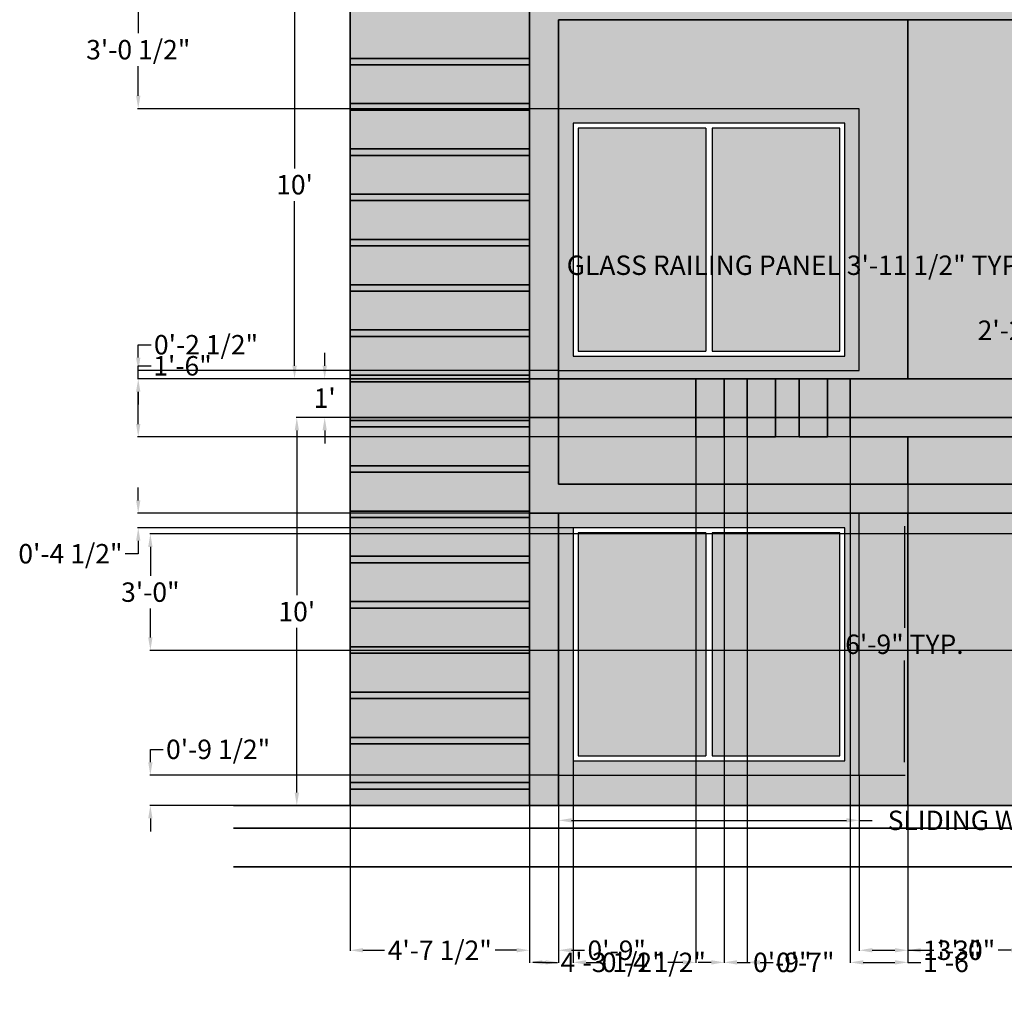
# Model space of a CAD drawing. Units: inches. Extents: x 23 to 640, y 58 to 516.
# Tile 1 of 4: x 23 to 328, y 58 to 359. Entities that reach past the tile are written whole.
import ezdxf

# ---------------------------------------------------------------- set-up
doc = ezdxf.new("R2010")
doc.units = ezdxf.units.IN
doc.header["$MEASUREMENT"] = 0
for name, color, linetype, lineweight in [('A-ANNO-DIMS', 2, 'Continuous', 18), ('A-ANNO-NPLT', 8, 'Continuous', 13), ('A-ELEV', 7, 'Continuous', 35), ('A-ELEV-PATT', 252, 'Continuous', 13), ('A-GLAZ', 4, 'Continuous', 25)]:
    doc.layers.add(name, color=color, linetype=linetype, lineweight=lineweight)
doc.styles.get("Standard").update_dxf_attribs({"font": 'arial.ttf'})
doc.dimstyles.get("Standard").update_dxf_attribs({"dimtxt": 6, "dimasz": 4, "dimexe": 0.18, "dimexo": 0.0625, "dimgap": 2, "dimtad": 0, "dimtih": 1, "dimtoh": 1, "dimdec": 0, "dimzin": 0, "dimdsep": 46, "dimlunit": 3, "dimtxsty": 'Standard', "dimcen": 2, "dimadec": 0, "dimazin": 0, "dimtfac": 1, "dimtdec": 0, "dimtofl": 0, "dimtmove": 0, "dimatfit": 3, "dimfxl": 1, "dimtolj": 1, "dimtzin": 0, "dimarcsym": 0})

# ---------------------------------------------------------------- blocks, each defined once
blk = doc.blocks.new('*D3')
at = {"layer": 'A-ANNO-DIMS', "color": 0, "lineweight": -2, "transparency": 16777216}
for p, q in [((125.37, 367.68), (108.09, 367.68)), ((108.27, 363.68), (108.27, 312.74)), ((108.27, 251.68), (108.27, 302.62)), ((125.37, 247.68), (108.09, 247.68))]:
    blk.add_line(p, q, dxfattribs=at)
at = {"layer": 'A-ANNO-DIMS', "color": 0, "transparency": 16777216}
for points in [[(107.61, 363.68), (108.94, 363.68), (108.27, 367.68)], [(107.61, 251.68), (108.94, 251.68), (108.27, 247.68)]]:
    blk.add_solid(points, dxfattribs=at)
at = {"layer": 'Defpoints', "color": 0, "transparency": 16777216}
for p in [(125.43, 367.68), (108.27, 247.68), (125.43, 247.68)]:
    blk.add_point(p, dxfattribs=at)
at = {"layer": 'A-ANNO-DIMS', "color": 0, "transparency": 16777216, "insert": (108.27, 307.68), "char_height": 6, "attachment_point": 5}
blk.add_mtext("\\A1;10'", dxfattribs=at)
blk = doc.blocks.new('*D4')
at = {"layer": 'A-ANNO-DIMS', "color": 0, "lineweight": -2, "transparency": 16777216}
for p, q in [((117.59, 251.68), (117.59, 255.68)), ((125.37, 247.68), (117.41, 247.68)), ((125.37, 235.68), (117.41, 235.68)), ((117.59, 231.68), (117.59, 227.68))]:
    blk.add_line(p, q, dxfattribs=at)
at = {"layer": 'A-ANNO-DIMS', "color": 0, "transparency": 16777216}
for points in [[(116.93, 251.68), (118.26, 251.68), (117.59, 247.68)], [(116.93, 231.68), (118.26, 231.68), (117.59, 235.68)]]:
    blk.add_solid(points, dxfattribs=at)
at = {"layer": 'Defpoints', "color": 0, "transparency": 16777216}
for p in [(125.43, 247.68), (117.59, 235.68), (125.43, 235.68)]:
    blk.add_point(p, dxfattribs=at)
at = {"layer": 'A-ANNO-DIMS', "color": 0, "transparency": 16777216, "insert": (117.59, 241.68), "char_height": 6, "attachment_point": 5}
blk.add_mtext("\\A1;1'", dxfattribs=at)
blk = doc.blocks.new('*D5')
at = {"layer": 'A-ANNO-DIMS', "color": 0, "lineweight": -2, "transparency": 16777216}
for p, q in [((125.37, 235.68), (108.79, 235.68)), ((108.97, 231.68), (108.97, 180.74)), ((108.97, 119.68), (108.97, 170.62)), ((125.37, 115.68), (108.79, 115.68))]:
    blk.add_line(p, q, dxfattribs=at)
at = {"layer": 'A-ANNO-DIMS', "color": 0, "transparency": 16777216}
for points in [[(108.31, 231.68), (109.64, 231.68), (108.97, 235.68)], [(108.31, 119.68), (109.64, 119.68), (108.97, 115.68)]]:
    blk.add_solid(points, dxfattribs=at)
at = {"layer": 'Defpoints', "color": 0, "transparency": 16777216}
for p in [(125.43, 235.68), (108.97, 115.68), (125.43, 115.68)]:
    blk.add_point(p, dxfattribs=at)
at = {"layer": 'A-ANNO-DIMS', "color": 0, "transparency": 16777216, "insert": (108.97, 175.68), "char_height": 6, "attachment_point": 5}
blk.add_mtext("\\A1;10'", dxfattribs=at)
blk = doc.blocks.new('WIN-SLIDING-2P')
for p, q in [((45.5, 75), (45.5, 6)), ((47.5, 75), (47.5, 6))]:
    blk.add_line(p, q)
for points in [[(93, 81), (0, 81), (0, 0), (93, 0)], [(88.5, 76.5), (4.5, 76.5), (4.5, 4.5), (88.5, 4.5)]]:
    blk.add_lwpolyline(points, close=True)
for points in [[(45.5, 75), (6, 75), (6, 6), (45.5, 6)], [(47.5, 6), (87, 6), (87, 75), (47.5, 75)]]:
    blk.add_lwpolyline(points)
blk = doc.blocks.new('*D13')
at = {"layer": 'A-ANNO-DIMS', "color": 0, "lineweight": -2, "transparency": 16777216}
for p, q in [((344.93, 282.78), (340.93, 282.78)), ((344.93, 275.74), (344.93, 282.96)), ((388.23, 282.78), (348.93, 282.78)), ((392.23, 275.74), (392.23, 282.96))]:
    blk.add_line(p, q, dxfattribs=at)
at = {"layer": 'A-ANNO-DIMS', "color": 0, "transparency": 16777216}
for points in [[(348.93, 283.44), (348.93, 282.11), (344.93, 282.78)], [(388.23, 283.44), (388.23, 282.11), (392.23, 282.78)]]:
    blk.add_solid(points, dxfattribs=at)
at = {"layer": 'Defpoints', "color": 0, "transparency": 16777216}
for p in [(344.93, 282.78), (344.93, 275.68), (392.23, 275.68)]:
    blk.add_point(p, dxfattribs=at)
at = {"layer": 'A-ANNO-DIMS', "color": 0, "transparency": 16777216, "insert": (263.39, 282.78), "char_height": 6, "attachment_point": 5}
blk.add_mtext('\\A1;GLASS RAILING PANEL 3\'-11 1/2" TYP.', dxfattribs=at)
blk = doc.blocks.new('*D14')
at = {"layer": 'A-ANNO-DIMS', "color": 0, "lineweight": -2, "transparency": 16777216}
for p, q in [((344.87, 275.68), (337.65, 275.68)), ((337.83, 271.68), (337.83, 267.7)), ((337.83, 253.68), (337.83, 257.67)), ((344.87, 249.68), (337.65, 249.68))]:
    blk.add_line(p, q, dxfattribs=at)
at = {"layer": 'A-ANNO-DIMS', "color": 0, "transparency": 16777216}
for points in [[(337.17, 271.68), (338.5, 271.68), (337.83, 275.68)], [(337.17, 253.68), (338.5, 253.68), (337.83, 249.68)]]:
    blk.add_solid(points, dxfattribs=at)
at = {"layer": 'Defpoints', "color": 0, "transparency": 16777216}
for p in [(344.93, 275.68), (337.83, 249.68), (344.93, 249.68)]:
    blk.add_point(p, dxfattribs=at)
at = {"layer": 'A-ANNO-DIMS', "color": 0, "transparency": 16777216, "insert": (337.83, 262.68), "char_height": 6, "attachment_point": 5}
blk.add_mtext('\\A1;2\'-2" TYP.', dxfattribs=at)
blk = doc.blocks.new('*D15')
at = {"layer": 'A-ANNO-DIMS', "color": 0, "lineweight": -2, "transparency": 16777216}
for p, q in [((189.93, 125), (189.93, 110.93)), ((282.93, 125), (282.93, 110.93)), ((193.93, 111.11), (278.93, 111.11)), ((282.93, 111.11), (286.93, 111.11))]:
    blk.add_line(p, q, dxfattribs=at)
at = {"layer": 'A-ANNO-DIMS', "color": 0, "transparency": 16777216}
for points in [[(193.93, 111.78), (193.93, 110.44), (189.93, 111.11)], [(278.93, 111.78), (278.93, 110.44), (282.93, 111.11)]]:
    blk.add_solid(points, dxfattribs=at)
at = {"layer": 'Defpoints', "color": 0, "transparency": 16777216}
for p in [(189.93, 125.06), (282.93, 125.06), (282.93, 111.11)]:
    blk.add_point(p, dxfattribs=at)
at = {"layer": 'A-ANNO-DIMS', "color": 0, "transparency": 16777216, "insert": (344.69, 111.11), "char_height": 6, "attachment_point": 5}
blk.add_mtext('\\A1;SLIDING WINDOW 7\'-9" TYP.', dxfattribs=at)
blk = doc.blocks.new('*D16')
at = {"layer": 'A-ANNO-DIMS', "color": 0, "lineweight": -2, "transparency": 16777216}
for p, q in [((282.99, 206.06), (297.06, 206.06)), ((296.88, 202.06), (296.88, 170.62)), ((296.88, 129.06), (296.88, 160.5)), ((282.99, 125.06), (297.06, 125.06))]:
    blk.add_line(p, q, dxfattribs=at)
at = {"layer": 'A-ANNO-DIMS', "color": 0, "transparency": 16777216}
for points in [[(296.21, 202.06), (297.55, 202.06), (296.88, 206.06)], [(296.21, 129.06), (297.55, 129.06), (296.88, 125.06)]]:
    blk.add_solid(points, dxfattribs=at)
at = {"layer": 'Defpoints', "color": 0, "transparency": 16777216}
for p in [(282.93, 206.06), (296.88, 206.06), (282.93, 125.06)]:
    blk.add_point(p, dxfattribs=at)
at = {"layer": 'A-ANNO-DIMS', "color": 0, "transparency": 16777216, "insert": (296.88, 165.56), "char_height": 6, "attachment_point": 5}
blk.add_mtext('\\A1;6\'-9" TYP.', dxfattribs=at)
blk = doc.blocks.new('*D23')
at = {"layer": 'A-ANNO-DIMS', "color": 0, "lineweight": -2, "transparency": 16777216}
for p, q in [((125.43, 115.62), (125.43, 70.75)), ((180.93, 115.62), (180.93, 70.75)), ((129.43, 70.93), (136.09, 70.93)), ((176.93, 70.93), (170.26, 70.93))]:
    blk.add_line(p, q, dxfattribs=at)
at = {"layer": 'A-ANNO-DIMS', "color": 0, "transparency": 16777216}
for points in [[(129.43, 71.6), (129.43, 70.26), (125.43, 70.93)], [(176.93, 71.6), (176.93, 70.26), (180.93, 70.93)]]:
    blk.add_solid(points, dxfattribs=at)
at = {"layer": 'Defpoints', "color": 0, "transparency": 16777216}
for p in [(125.43, 115.68), (180.93, 115.68), (180.93, 70.93)]:
    blk.add_point(p, dxfattribs=at)
at = {"layer": 'A-ANNO-DIMS', "color": 0, "transparency": 16777216, "insert": (153.18, 70.93), "char_height": 6, "attachment_point": 5}
blk.add_mtext('\\A1;4\'-7 1/2"', dxfattribs=at)
blk = doc.blocks.new('*D24')
at = {"layer": 'A-ANNO-DIMS', "color": 0, "lineweight": -2, "transparency": 16777216}
for p, q in [((180.93, 115.62), (180.93, 70.75)), ((189.93, 115.62), (189.93, 70.75)), ((176.93, 70.93), (172.93, 70.93)), ((193.93, 70.93), (197.93, 70.93))]:
    blk.add_line(p, q, dxfattribs=at)
at = {"layer": 'A-ANNO-DIMS', "color": 0, "transparency": 16777216}
for points in [[(176.93, 71.6), (176.93, 70.26), (180.93, 70.93)], [(193.93, 71.6), (193.93, 70.26), (189.93, 70.93)]]:
    blk.add_solid(points, dxfattribs=at)
at = {"layer": 'Defpoints', "color": 0, "transparency": 16777216}
for p in [(180.93, 115.68), (189.93, 115.68), (189.93, 70.93)]:
    blk.add_point(p, dxfattribs=at)
at = {"layer": 'A-ANNO-DIMS', "color": 0, "transparency": 16777216, "insert": (207.9, 70.93), "char_height": 6, "attachment_point": 5}
blk.add_mtext('\\A1;0\'-9"', dxfattribs=at)
blk = doc.blocks.new('*D25')
at = {"layer": 'A-ANNO-DIMS', "color": 0, "lineweight": -2, "transparency": 16777216}
for p, q in [((282.93, 125), (282.93, 70.75)), ((297.93, 115.62), (297.93, 70.75)), ((286.93, 70.93), (293.93, 70.93)), ((297.93, 70.93), (301.93, 70.93))]:
    blk.add_line(p, q, dxfattribs=at)
at = {"layer": 'A-ANNO-DIMS', "color": 0, "transparency": 16777216}
for points in [[(286.93, 71.6), (286.93, 70.26), (282.93, 70.93)], [(293.93, 71.6), (293.93, 70.26), (297.93, 70.93)]]:
    blk.add_solid(points, dxfattribs=at)
at = {"layer": 'Defpoints', "color": 0, "transparency": 16777216}
for p in [(282.93, 125.06), (297.93, 115.68), (297.93, 70.93)]:
    blk.add_point(p, dxfattribs=at)
at = {"layer": 'A-ANNO-DIMS', "color": 0, "transparency": 16777216, "insert": (311.62, 70.93), "char_height": 6, "attachment_point": 5}
blk.add_mtext('\\A1;1\'-3"', dxfattribs=at)
blk = doc.blocks.new('*D26')
at = {"layer": 'A-ANNO-DIMS', "color": 0, "lineweight": -2, "transparency": 16777216}
for p, q in [((297.93, 115.62), (297.93, 70.75)), ((333.93, 115.62), (333.93, 70.75)), ((301.93, 70.93), (305.96, 70.93)), ((329.93, 70.93), (325.9, 70.93))]:
    blk.add_line(p, q, dxfattribs=at)
at = {"layer": 'A-ANNO-DIMS', "color": 0, "transparency": 16777216}
for points in [[(301.93, 71.6), (301.93, 70.26), (297.93, 70.93)], [(329.93, 71.6), (329.93, 70.26), (333.93, 70.93)]]:
    blk.add_solid(points, dxfattribs=at)
at = {"layer": 'Defpoints', "color": 0, "transparency": 16777216}
for p in [(297.93, 115.68), (333.93, 115.68), (333.93, 70.93)]:
    blk.add_point(p, dxfattribs=at)
at = {"layer": 'A-ANNO-DIMS', "color": 0, "transparency": 16777216, "insert": (315.93, 70.93), "char_height": 6, "attachment_point": 5}
blk.add_mtext('\\A1;3\'-0"', dxfattribs=at)
blk = doc.blocks.new('*D34')
at = {"layer": 'A-ANNO-DIMS', "color": 0, "lineweight": -2, "transparency": 16777216}
for p, q in [((63.68, 129.06), (63.68, 133.06)), ((63.68, 133.06), (67.68, 133.06)), ((189.87, 125.06), (63.5, 125.06)), ((189.87, 115.68), (63.5, 115.68)), ((63.68, 111.68), (63.68, 107.68))]:
    blk.add_line(p, q, dxfattribs=at)
at = {"layer": 'A-ANNO-DIMS', "color": 0, "transparency": 16777216}
for points in [[(63.01, 129.06), (64.35, 129.06), (63.68, 125.06)], [(63.01, 111.68), (64.35, 111.68), (63.68, 115.68)]]:
    blk.add_solid(points, dxfattribs=at)
at = {"layer": 'Defpoints', "color": 0, "transparency": 16777216}
for p in [(63.68, 125.06), (189.93, 125.06), (189.93, 115.68)]:
    blk.add_point(p, dxfattribs=at)
at = {"layer": 'A-ANNO-DIMS', "color": 0, "transparency": 16777216, "insert": (84.64, 133.06), "char_height": 6, "attachment_point": 5}
blk.add_mtext('\\A1;0\'-9 1/2"', dxfattribs=at)
blk = doc.blocks.new('*D37')
at = {"layer": 'A-ANNO-DIMS', "color": 0, "lineweight": -2, "transparency": 16777216}
for p, q in [((363.87, 199.68), (63.5, 199.68)), ((63.68, 195.68), (63.68, 186.75)), ((63.68, 167.68), (63.68, 176.62)), ((363.87, 163.68), (63.5, 163.68))]:
    blk.add_line(p, q, dxfattribs=at)
at = {"layer": 'A-ANNO-DIMS', "color": 0, "transparency": 16777216}
for points in [[(63.01, 195.68), (64.35, 195.68), (63.68, 199.68)], [(63.01, 167.68), (64.35, 167.68), (63.68, 163.68)]]:
    blk.add_solid(points, dxfattribs=at)
at = {"layer": 'Defpoints', "color": 0, "transparency": 16777216}
for p in [(63.68, 199.68), (363.93, 199.68), (363.93, 163.68)]:
    blk.add_point(p, dxfattribs=at)
at = {"layer": 'A-ANNO-DIMS', "color": 0, "transparency": 16777216, "insert": (63.68, 181.68), "char_height": 6, "attachment_point": 5}
blk.add_mtext('\\A1;3\'-0"', dxfattribs=at)
blk = doc.blocks.new('*D52')
at = {"layer": 'A-ANNO-DIMS', "color": 0, "lineweight": -2, "transparency": 16777216}
for p, q in [((280.13, 229.62), (280.13, 67)), ((297.93, 229.62), (297.93, 67)), ((284.13, 67.18), (293.93, 67.18)), ((297.93, 67.18), (301.93, 67.18))]:
    blk.add_line(p, q, dxfattribs=at)
at = {"layer": 'A-ANNO-DIMS', "color": 0, "transparency": 16777216}
for points in [[(284.13, 67.85), (284.13, 66.51), (280.13, 67.18)], [(293.93, 67.85), (293.93, 66.51), (297.93, 67.18)]]:
    blk.add_solid(points, dxfattribs=at)
at = {"layer": 'Defpoints', "color": 0, "transparency": 16777216}
for p in [(280.13, 229.68), (297.93, 229.68), (297.93, 67.18)]:
    blk.add_point(p, dxfattribs=at)
at = {"layer": 'A-ANNO-DIMS', "color": 0, "transparency": 16777216, "insert": (311.62, 67.18), "char_height": 6, "attachment_point": 5}
blk.add_mtext('\\A1;1\'-6"', dxfattribs=at)
blk = doc.blocks.new('*D53')
at = {"layer": 'A-ANNO-DIMS', "color": 0, "lineweight": -2, "transparency": 16777216}
for p, q in [((59.93, 247.68), (59.93, 251.68)), ((59.93, 251.68), (63.93, 251.68)), ((280.07, 247.68), (59.75, 247.68)), ((59.93, 233.68), (59.93, 243.68)), ((280.07, 229.68), (59.75, 229.68))]:
    blk.add_line(p, q, dxfattribs=at)
at = {"layer": 'A-ANNO-DIMS', "color": 0, "transparency": 16777216}
for points in [[(59.26, 243.68), (60.6, 243.68), (59.93, 247.68)], [(59.26, 233.68), (60.6, 233.68), (59.93, 229.68)]]:
    blk.add_solid(points, dxfattribs=at)
at = {"layer": 'Defpoints', "color": 0, "transparency": 16777216}
for p in [(59.93, 247.68), (280.13, 247.68), (280.13, 229.68)]:
    blk.add_point(p, dxfattribs=at)
at = {"layer": 'A-ANNO-DIMS', "color": 0, "transparency": 16777216, "insert": (73.62, 251.68), "char_height": 6, "attachment_point": 5}
blk.add_mtext('\\A1;1\'-6"', dxfattribs=at)
blk = doc.blocks.new('*D54')
at = {"layer": 'A-ANNO-DIMS', "color": 0, "lineweight": -2, "transparency": 16777216}
for p, q in [((180.93, 232.7), (180.93, 67)), ((232.34, 229.62), (232.34, 67)), ((184.93, 67.18), (189.55, 67.18)), ((228.34, 67.18), (223.72, 67.18))]:
    blk.add_line(p, q, dxfattribs=at)
at = {"layer": 'A-ANNO-DIMS', "color": 0, "transparency": 16777216}
for points in [[(184.93, 67.85), (184.93, 66.51), (180.93, 67.18)], [(228.34, 67.85), (228.34, 66.51), (232.34, 67.18)]]:
    blk.add_solid(points, dxfattribs=at)
at = {"layer": 'Defpoints', "color": 0, "transparency": 16777216}
for p in [(180.93, 232.76), (232.34, 229.68), (232.34, 67.18)]:
    blk.add_point(p, dxfattribs=at)
at = {"layer": 'A-ANNO-DIMS', "color": 0, "transparency": 16777216, "insert": (206.63, 67.18), "char_height": 6, "attachment_point": 5}
blk.add_mtext('\\A1;4\'-3 1/2"', dxfattribs=at)
blk = doc.blocks.new('*D55')
at = {"layer": 'A-ANNO-DIMS', "color": 0, "lineweight": -2, "transparency": 16777216}
for p, q in [((232.34, 229.62), (232.34, 67)), ((241.13, 229.62), (241.13, 67)), ((228.34, 67.18), (224.34, 67.18)), ((245.13, 67.18), (249.13, 67.18))]:
    blk.add_line(p, q, dxfattribs=at)
at = {"layer": 'A-ANNO-DIMS', "color": 0, "transparency": 16777216}
for points in [[(228.34, 67.85), (228.34, 66.51), (232.34, 67.18)], [(245.13, 67.85), (245.13, 66.51), (241.13, 67.18)]]:
    blk.add_solid(points, dxfattribs=at)
at = {"layer": 'Defpoints', "color": 0, "transparency": 16777216}
for p in [(232.34, 229.68), (241.13, 229.68), (241.13, 67.18)]:
    blk.add_point(p, dxfattribs=at)
at = {"layer": 'A-ANNO-DIMS', "color": 0, "transparency": 16777216, "insert": (259.11, 67.18), "char_height": 6, "attachment_point": 5}
blk.add_mtext('\\A1;0\'-9"', dxfattribs=at)
blk = doc.blocks.new('*D56')
at = {"layer": 'A-ANNO-DIMS', "color": 0, "lineweight": -2, "transparency": 16777216}
for p, q in [((241.13, 229.62), (241.13, 67)), ((248.24, 229.62), (248.24, 67)), ((237.13, 67.18), (233.13, 67.18)), ((252.24, 67.18), (256.24, 67.18))]:
    blk.add_line(p, q, dxfattribs=at)
at = {"layer": 'A-ANNO-DIMS', "color": 0, "transparency": 16777216}
for points in [[(237.13, 67.85), (237.13, 66.51), (241.13, 67.18)], [(252.24, 67.85), (252.24, 66.51), (248.24, 67.18)]]:
    blk.add_solid(points, dxfattribs=at)
at = {"layer": 'Defpoints', "color": 0, "transparency": 16777216}
for p in [(241.13, 229.68), (248.24, 229.68), (248.24, 67.18)]:
    blk.add_point(p, dxfattribs=at)
at = {"layer": 'A-ANNO-DIMS', "color": 0, "transparency": 16777216, "insert": (266.21, 67.18), "char_height": 6, "attachment_point": 5}
blk.add_mtext('\\A1;0\'-7"', dxfattribs=at)
blk = doc.blocks.new('*D57')
at = {"layer": 'A-ANNO-DIMS', "color": 0, "lineweight": -2, "transparency": 16777216}
for p, q in [((59.93, 254.2), (59.93, 258.2)), ((59.93, 258.2), (63.93, 258.2)), ((189.87, 250.2), (59.75, 250.2)), ((125.37, 247.68), (59.75, 247.68)), ((59.93, 243.68), (59.93, 239.68))]:
    blk.add_line(p, q, dxfattribs=at)
at = {"layer": 'A-ANNO-DIMS', "color": 0, "transparency": 16777216}
for points in [[(59.26, 254.2), (60.6, 254.2), (59.93, 250.2)], [(59.26, 243.68), (60.6, 243.68), (59.93, 247.68)]]:
    blk.add_solid(points, dxfattribs=at)
at = {"layer": 'Defpoints', "color": 0, "transparency": 16777216}
for p in [(59.93, 250.2), (189.93, 250.2), (125.43, 247.68)]:
    blk.add_point(p, dxfattribs=at)
at = {"layer": 'A-ANNO-DIMS', "color": 0, "transparency": 16777216, "insert": (80.89, 258.2), "char_height": 6, "attachment_point": 5}
blk.add_mtext('\\A1;0\'-2 1/2"', dxfattribs=at)
blk = doc.blocks.new('*D58')
at = {"layer": 'A-ANNO-DIMS', "color": 0, "lineweight": -2, "transparency": 16777216}
for p, q in [((297.87, 367.68), (59.75, 367.68)), ((59.93, 363.68), (59.93, 354.54)), ((59.93, 335.2), (59.93, 344.34)), ((282.87, 331.2), (59.75, 331.2))]:
    blk.add_line(p, q, dxfattribs=at)
at = {"layer": 'A-ANNO-DIMS', "color": 0, "transparency": 16777216}
for points in [[(59.26, 363.68), (60.6, 363.68), (59.93, 367.68)], [(59.26, 335.2), (60.6, 335.2), (59.93, 331.2)]]:
    blk.add_solid(points, dxfattribs=at)
at = {"layer": 'Defpoints', "color": 0, "transparency": 16777216}
for p in [(59.93, 367.68), (297.93, 367.68), (282.93, 331.2)]:
    blk.add_point(p, dxfattribs=at)
at = {"layer": 'A-ANNO-DIMS', "color": 0, "transparency": 16777216, "insert": (59.93, 349.44), "char_height": 6, "attachment_point": 5}
blk.add_mtext('\\A1;3\'-0 1/2"', dxfattribs=at)
blk = doc.blocks.new('*D61')
at = {"layer": 'A-ANNO-DIMS', "color": 0, "lineweight": -2, "transparency": 16777216}
for p, q in [((189.93, 206), (189.93, 67)), ((194.43, 201.5), (194.43, 67)), ((185.93, 67.18), (181.93, 67.18)), ((198.43, 67.18), (202.43, 67.18))]:
    blk.add_line(p, q, dxfattribs=at)
at = {"layer": 'A-ANNO-DIMS', "color": 0, "transparency": 16777216}
for points in [[(185.93, 67.85), (185.93, 66.51), (189.93, 67.18)], [(198.43, 67.85), (198.43, 66.51), (194.43, 67.18)]]:
    blk.add_solid(points, dxfattribs=at)
at = {"layer": 'Defpoints', "color": 0, "transparency": 16777216}
for p in [(189.93, 206.06), (194.43, 201.56), (194.43, 67.18)]:
    blk.add_point(p, dxfattribs=at)
at = {"layer": 'A-ANNO-DIMS', "color": 0, "transparency": 16777216, "insert": (219.39, 67.18), "char_height": 6, "attachment_point": 5}
blk.add_mtext('\\A1;0\'-4 1/2"', dxfattribs=at)
blk = doc.blocks.new('*D62')
at = {"layer": 'A-ANNO-DIMS', "color": 0, "lineweight": -2, "transparency": 16777216}
for p, q in [((59.93, 210.06), (59.93, 214.06)), ((189.87, 206.06), (59.75, 206.06)), ((194.37, 201.56), (59.75, 201.56)), ((59.93, 197.56), (59.93, 193.56)), ((59.93, 193.56), (55.93, 193.56))]:
    blk.add_line(p, q, dxfattribs=at)
at = {"layer": 'A-ANNO-DIMS', "color": 0, "transparency": 16777216}
for points in [[(59.26, 210.06), (60.6, 210.06), (59.93, 206.06)], [(59.26, 197.56), (60.6, 197.56), (59.93, 201.56)]]:
    blk.add_solid(points, dxfattribs=at)
at = {"layer": 'Defpoints', "color": 0, "transparency": 16777216}
for p in [(189.93, 206.06), (59.93, 201.56), (194.43, 201.56)]:
    blk.add_point(p, dxfattribs=at)
at = {"layer": 'A-ANNO-DIMS', "color": 0, "transparency": 16777216, "insert": (38.96, 193.56), "char_height": 6, "attachment_point": 5}
blk.add_mtext('\\A1;0\'-4 1/2"', dxfattribs=at)

msp = doc.modelspace()

# ---------------------------------------------------------------- hatches: boundary and pattern name
at = {"layer": 'A-ELEV-PATT'}
h = msp.add_hatch(color=256, dxfattribs=at)
h.dxf.hatch_style = 1
h.paths.add_polyline_path([(180.93, 120.76), (125.43, 120.76), (125.43, 115.68), (180.93, 115.68)])
h.paths.add_polyline_path([(180.93, 134.76), (125.43, 134.76), (125.43, 122.76), (180.93, 122.76)])
h.paths.add_polyline_path([(180.93, 148.76), (125.43, 148.76), (125.43, 136.76), (180.93, 136.76)])
h.paths.add_polyline_path([(180.93, 162.76), (125.43, 162.76), (125.43, 150.76), (180.93, 150.76)])
h.paths.add_polyline_path([(180.93, 176.76), (125.43, 176.76), (125.43, 164.76), (180.93, 164.76)])
h.paths.add_polyline_path([(180.93, 190.76), (125.43, 190.76), (125.43, 178.76), (180.93, 178.76)])
h.paths.add_polyline_path([(180.93, 204.76), (125.43, 204.76), (125.43, 192.76), (180.93, 192.76)])
h.paths.add_polyline_path([(180.93, 218.76), (125.43, 218.76), (125.43, 206.76), (180.93, 206.76)])
h.paths.add_polyline_path([(180.93, 232.76), (125.43, 232.76), (125.43, 220.76), (180.93, 220.76)])
h.paths.add_polyline_path([(180.93, 246.76), (125.43, 246.76), (125.43, 235.68), (180.93, 235.68)])
h.paths.add_polyline_path([(180.93, 235.68), (125.43, 235.68), (125.43, 234.76), (180.93, 234.76)])
h.paths.add_polyline_path([(180.93, 260.76), (125.43, 260.76), (125.43, 248.76), (180.93, 248.76)])
h.paths.add_polyline_path([(180.93, 274.76), (125.43, 274.76), (125.43, 262.76), (180.93, 262.76)])
h.paths.add_polyline_path([(180.93, 288.76), (125.43, 288.76), (125.43, 276.76), (180.93, 276.76)])
h.paths.add_polyline_path([(180.93, 302.76), (125.43, 302.76), (125.43, 290.76), (180.93, 290.76)])
h.paths.add_polyline_path([(180.93, 316.76), (125.43, 316.76), (125.43, 304.76), (180.93, 304.76)])
h.paths.add_polyline_path([(180.93, 330.76), (125.43, 330.76), (125.43, 318.76), (180.93, 318.76)])
h.paths.add_polyline_path([(180.93, 344.76), (125.43, 344.76), (125.43, 332.76), (180.93, 332.76)])
h.paths.add_polyline_path([(180.93, 358.76), (125.43, 358.76), (125.43, 346.76), (180.93, 346.76)])
h.paths.add_polyline_path([(180.93, 367.68), (125.43, 367.68), (125.43, 360.76), (180.93, 360.76)])
h.paths.add_polyline_path([(297.93, 372.76), (125.43, 372.76), (125.43, 367.68), (180.93, 367.68), (297.93, 367.68)])
h.paths.add_polyline_path([(297.93, 379.68), (125.43, 379.68), (125.43, 374.76), (297.93, 374.76)])
h.paths.add_polyline_path([(297.93, 386.76), (125.43, 386.76), (125.43, 379.68), (297.93, 379.68)])
h.paths.add_polyline_path([(297.93, 400.76), (125.43, 400.76), (125.43, 388.76), (297.93, 388.76)])
h.paths.add_polyline_path([(297.93, 414.76), (125.43, 414.76), (125.43, 402.76), (297.93, 402.76)])
h.paths.add_polyline_path([(297.93, 433.68), (125.43, 433.68), (125.43, 430.76), (297.93, 430.76)])
h.paths.add_polyline_path([(386.63, 372.76), (333.93, 372.76), (333.93, 367.68), (386.63, 367.68)])
h.paths.add_polyline_path([(386.63, 379.68), (333.93, 379.68), (333.93, 374.76), (386.63, 374.76)])
h.paths.add_polyline_path([(386.63, 386.76), (333.93, 386.76), (333.93, 379.68), (386.63, 379.68)])
h.paths.add_polyline_path([(386.63, 400.76), (333.93, 400.76), (333.93, 388.76), (386.63, 388.76)])
h.paths.add_polyline_path([(386.63, 414.76), (333.93, 414.76), (333.93, 402.76), (386.63, 402.76)])
h.paths.add_polyline_path([(386.63, 428.76), (333.93, 428.76), (333.93, 416.76), (386.63, 416.76)])
h.paths.add_polyline_path([(386.63, 433.68), (333.93, 433.68), (333.93, 430.76), (386.63, 430.76)])
h = msp.add_hatch(color=256, dxfattribs=at)
h.dxf.hatch_style = 1
h.paths.add_polyline_path([(333.93, 433.68), (297.93, 433.68), (297.93, 379.68), (333.93, 379.68)])
h.paths.add_polyline_path([(333.93, 379.68), (297.93, 379.68), (297.93, 367.68), (333.93, 367.68)])
h.paths.add_polyline_path([(333.93, 358.68), (297.93, 358.68), (297.93, 247.68), (333.93, 247.68)])
h.paths.add_polyline_path([(333.93, 229.68), (297.93, 229.68), (297.93, 215.06), (333.93, 215.06)])
h.paths.add_polyline_path([(333.93, 206.06), (297.93, 206.06), (297.93, 115.68), (333.93, 115.68)])
h = msp.add_hatch(color=256, dxfattribs=at)
h.dxf.hatch_style = 1
h.paths.add_polyline_path([(180.93, 122.76), (125.43, 122.76), (125.43, 120.76), (180.93, 120.76)])
h.paths.add_polyline_path([(180.93, 136.76), (125.43, 136.76), (125.43, 134.76), (180.93, 134.76)])
h.paths.add_polyline_path([(180.93, 150.76), (125.43, 150.76), (125.43, 148.76), (180.93, 148.76)])
h.paths.add_polyline_path([(180.93, 164.76), (125.43, 164.76), (125.43, 162.76), (180.93, 162.76)])
h.paths.add_polyline_path([(180.93, 178.76), (125.43, 178.76), (125.43, 176.76), (180.93, 176.76)])
h.paths.add_polyline_path([(180.93, 192.76), (125.43, 192.76), (125.43, 190.76), (180.93, 190.76)])
h.paths.add_polyline_path([(180.93, 206.76), (125.43, 206.76), (125.43, 204.76), (180.93, 204.76)])
h.paths.add_polyline_path([(180.93, 220.76), (125.43, 220.76), (125.43, 218.76), (180.93, 218.76)])
h.paths.add_polyline_path([(180.93, 234.76), (125.43, 234.76), (125.43, 232.76), (180.93, 232.76)])
h.paths.add_polyline_path([(180.93, 247.68), (125.43, 247.68), (125.43, 246.76), (180.93, 246.76)])
h.paths.add_polyline_path([(180.93, 248.76), (125.43, 248.76), (125.43, 247.68), (180.93, 247.68)])
h.paths.add_polyline_path([(180.93, 262.76), (125.43, 262.76), (125.43, 260.76), (180.93, 260.76)])
h.paths.add_polyline_path([(180.93, 276.76), (125.43, 276.76), (125.43, 274.76), (180.93, 274.76)])
h.paths.add_polyline_path([(180.93, 290.76), (125.43, 290.76), (125.43, 288.76), (180.93, 288.76)])
h.paths.add_polyline_path([(180.93, 304.76), (125.43, 304.76), (125.43, 302.76), (180.93, 302.76)])
h.paths.add_polyline_path([(180.93, 318.76), (125.43, 318.76), (125.43, 316.76), (180.93, 316.76)])
h.paths.add_polyline_path([(180.93, 332.76), (125.43, 332.76), (125.43, 330.76), (180.93, 330.76)])
h.paths.add_polyline_path([(180.93, 346.76), (125.43, 346.76), (125.43, 344.76), (180.93, 344.76)])
h.paths.add_polyline_path([(180.93, 360.76), (125.43, 360.76), (125.43, 358.76), (180.93, 358.76)])
h.paths.add_polyline_path([(297.93, 374.76), (125.43, 374.76), (125.43, 372.76), (297.93, 372.76)])
h.paths.add_polyline_path([(297.93, 388.76), (125.43, 388.76), (125.43, 386.76), (297.93, 386.76)])
h.paths.add_polyline_path([(297.93, 402.76), (125.43, 402.76), (125.43, 400.76), (297.93, 400.76)])
h.paths.add_polyline_path([(297.93, 416.76), (125.43, 416.76), (125.43, 414.76), (297.93, 414.76)])
h.paths.add_polyline_path([(297.93, 430.76), (125.43, 430.76), (125.43, 428.76), (297.93, 428.76)])
h.paths.add_polyline_path([(386.63, 374.76), (333.93, 374.76), (333.93, 372.76), (386.63, 372.76)])
h.paths.add_polyline_path([(386.63, 388.76), (333.93, 388.76), (333.93, 386.76), (386.63, 386.76)])
h.paths.add_polyline_path([(386.63, 402.76), (333.93, 402.76), (333.93, 400.76), (386.63, 400.76)])
h.paths.add_polyline_path([(386.63, 416.76), (333.93, 416.76), (333.93, 414.76), (386.63, 414.76)])
h.paths.add_polyline_path([(386.63, 430.76), (333.93, 430.76), (333.93, 428.76), (386.63, 428.76)])
h = msp.add_hatch(color=256, dxfattribs=at)
h.dxf.hatch_style = 1
h.paths.add_polyline_path([(371.93, 367.68), (180.93, 367.68), (180.93, 247.68), (189.93, 247.68), (189.93, 358.68), (371.93, 358.68)])
h.paths.add_polyline_path([(189.93, 247.68), (180.93, 247.68), (180.93, 235.68), (189.93, 235.68)])
h.paths.add_polyline_path([(189.93, 235.68), (180.93, 235.68), (180.93, 206.06), (333.93, 206.06), (351.93, 206.06), (351.93, 211.68), (351.93, 215.06), (189.93, 215.06)])
h.paths.add_polyline_path([(551.13, 247.68), (280.13, 247.68), (280.13, 235.68), (551.13, 235.68)])
h.paths.add_polyline_path([(551.13, 235.68), (280.13, 235.68), (280.13, 229.68), (551.13, 229.68)])
h = msp.add_hatch(color=256, dxfattribs=at)
h.set_gradient(color1=(147, 149, 152), color2=(199, 200, 202), name='CYLINDER')
h.paths.add_polyline_path([(297.93, 358.68), (189.93, 358.68), (189.93, 331.2), (282.93, 331.2), (282.93, 250.2), (189.93, 250.2), (189.93, 247.68), (297.93, 247.68)])
h.paths.add_polyline_path([(232.34, 235.68), (189.93, 235.68), (189.93, 215.06), (297.93, 215.06), (297.93, 229.68), (280.13, 229.68), (280.13, 235.68), (273.12, 235.68), (273.12, 229.68), (264.33, 229.68), (264.33, 235.68), (257.03, 235.68), (257.03, 229.68), (248.24, 229.68), (248.24, 235.68), (241.13, 235.68), (241.13, 229.68), (232.34, 229.68)])
h.paths.add_polyline_path([(232.34, 247.68), (189.93, 247.68), (189.93, 235.68), (232.34, 235.68)])
h.paths.add_polyline_path([(248.24, 247.68), (241.13, 247.68), (241.13, 235.68), (248.24, 235.68)])
h.paths.add_polyline_path([(264.33, 247.68), (257.03, 247.68), (257.03, 235.68), (264.33, 235.68)])
h.paths.add_polyline_path([(280.13, 247.68), (273.12, 247.68), (273.12, 235.68), (280.13, 235.68)])
h.paths.add_polyline_path([(297.93, 206.06), (282.93, 206.06), (282.93, 125.06), (189.93, 125.06), (189.93, 115.68), (297.93, 115.68)])
h.paths.add_polyline_path([(189.93, 206.06), (180.93, 206.06), (180.93, 115.68), (189.93, 115.68)])
h = msp.add_hatch(color=256, dxfattribs=at)
h.set_gradient(color1=(153, 76, 76), color2=(147, 149, 152), name='SPHERICAL')
h.paths.add_polyline_path([(189.93, 331.2), (189.93, 250.2), (282.93, 250.2), (282.93, 331.2)])
h.paths.add_polyline_path([(194.43, 326.7), (278.43, 326.7), (278.43, 254.7), (194.43, 254.7)], flags=16)
h.paths.add_polyline_path([(195.93, 325.2), (235.43, 325.2), (235.43, 256.2), (195.93, 256.2)], flags=0)
h.paths.add_polyline_path([(237.43, 325.2), (276.93, 325.2), (276.93, 256.2), (237.43, 256.2)], flags=0)
h = msp.add_hatch(color=256, dxfattribs=at)
h.set_gradient(color1=(255, 255, 255), color2=(173, 221, 247), name='INVSPHERICAL')
h.paths.add_polyline_path([(195.93, 256.2), (235.43, 256.2), (235.43, 325.2), (195.93, 325.2)])
h = msp.add_hatch(color=256, dxfattribs=at)
h.set_gradient(color1=(255, 255, 255), color2=(173, 221, 247), name='INVSPHERICAL')
h.paths.add_polyline_path([(237.43, 256.2), (276.93, 256.2), (276.93, 325.2), (237.43, 325.2)])
h = msp.add_hatch(color=256, dxfattribs=at)
h.paths.add_polyline_path([(273.12, 247.68), (264.33, 247.68), (264.33, 235.68), (273.12, 235.68)])
h.paths.add_polyline_path([(257.03, 247.68), (248.24, 247.68), (248.24, 235.68), (257.03, 235.68)])
h.paths.add_polyline_path([(241.13, 247.68), (232.34, 247.68), (232.34, 235.68), (241.13, 235.68)])
h.paths.add_polyline_path([(241.13, 235.68), (232.34, 235.68), (232.34, 229.68), (241.13, 229.68)])
h.paths.add_polyline_path([(257.03, 235.68), (248.24, 235.68), (248.24, 229.68), (257.03, 229.68)])
h.paths.add_polyline_path([(273.12, 235.68), (264.33, 235.68), (264.33, 229.68), (273.12, 229.68)])
h = msp.add_hatch(color=256, dxfattribs=at)
h.set_gradient(color1=(153, 76, 76), color2=(147, 149, 152), name='SPHERICAL')
h.paths.add_polyline_path([(189.93, 206.06), (189.93, 125.06), (282.93, 125.06), (282.93, 206.06)])
h.paths.add_polyline_path([(194.43, 201.56), (278.43, 201.56), (278.43, 129.56), (194.43, 129.56)], flags=16)
h.paths.add_polyline_path([(195.93, 200.06), (235.43, 200.06), (235.43, 131.06), (195.93, 131.06)], flags=0)
h.paths.add_polyline_path([(237.43, 200.06), (276.93, 200.06), (276.93, 131.06), (237.43, 131.06)], flags=0)
h = msp.add_hatch(color=256, dxfattribs=at)
h.set_gradient(color1=(255, 255, 255), color2=(173, 221, 247), name='INVSPHERICAL')
h.paths.add_polyline_path([(195.93, 131.06), (235.43, 131.06), (235.43, 200.06), (195.93, 200.06)])
h = msp.add_hatch(color=256, dxfattribs=at)
h.set_gradient(color1=(255, 255, 255), color2=(173, 221, 247), name='INVSPHERICAL')
h.paths.add_polyline_path([(237.43, 131.06), (276.93, 131.06), (276.93, 200.06), (237.43, 200.06)])

# ---------------------------------------------------------------- linework, layer by layer
at = {"layer": 'A-ANNO-NPLT'}
for p in [(125.43, 349.68), (125.43, 337.68), (125.43, 325.68), (125.43, 313.68), (125.43, 301.68), (125.43, 289.68), (125.43, 277.68), (125.43, 265.68), (125.43, 253.68), (125.43, 241.68), (125.43, 229.68), (125.43, 217.68), (125.43, 205.68), (125.43, 193.68), (125.43, 181.68), (125.43, 169.68), (125.43, 157.68), (125.43, 145.68), (125.43, 133.68), (125.43, 121.68)]:
    msp.add_point(p, dxfattribs=at)
at = {"layer": 'A-ELEV'}
for p, q in [((125.43, 115.68), (125.43, 433.68)), ((180.93, 115.68), (180.93, 367.68)), ((189.93, 358.68), (371.93, 358.68)), ((189.93, 215.06), (189.93, 358.68)), ((297.93, 358.68), (297.93, 247.68)), ((125.43, 346.76), (180.93, 346.76)), ((125.43, 344.76), (180.93, 344.76)), ((125.43, 332.76), (180.93, 332.76)), ((125.43, 330.76), (180.93, 330.76)), ((125.43, 318.76), (180.93, 318.76)), ((125.43, 316.76), (180.93, 316.76)), ((125.43, 304.76), (180.93, 304.76)), ((125.43, 302.76), (180.93, 302.76)), ((125.43, 290.76), (180.93, 290.76)), ((125.43, 288.76), (180.93, 288.76)), ((125.43, 276.76), (180.93, 276.76)), ((125.43, 274.76), (180.93, 274.76)), ((125.43, 262.76), (180.93, 262.76)), ((125.43, 260.76), (180.93, 260.76)), ((125.43, 248.76), (180.93, 248.76)), ((125.43, 247.68), (551.13, 247.68)), ((125.43, 246.76), (180.93, 246.76)), ((280.13, 247.68), (551.13, 247.68)), ((280.13, 247.68), (280.13, 229.68)), ((125.43, 235.68), (551.13, 235.68)), ((125.43, 234.76), (180.93, 234.76)), ((125.43, 232.76), (180.93, 232.76)), ((232.34, 229.68), (241.13, 229.68)), ((248.24, 229.68), (257.03, 229.68)), ((264.33, 229.68), (273.12, 229.68)), ((280.13, 229.68), (551.13, 229.68)), ((297.93, 229.68), (297.93, 215.06)), ((125.43, 220.76), (180.93, 220.76)), ((125.43, 218.76), (180.93, 218.76)), ((351.93, 215.06), (189.93, 215.06)), ((125.43, 206.76), (180.93, 206.76)), ((125.43, 204.76), (180.93, 204.76)), ((180.93, 206.06), (333.93, 206.06)), ((189.93, 115.68), (189.93, 206.06)), ((297.93, 206.06), (297.93, 115.68)), ((125.43, 192.76), (180.93, 192.76)), ((125.43, 190.76), (180.93, 190.76)), ((125.43, 178.76), (180.93, 178.76)), ((125.43, 176.76), (180.93, 176.76)), ((125.43, 164.76), (180.93, 164.76)), ((125.43, 162.76), (180.93, 162.76)), ((125.43, 150.76), (180.93, 150.76)), ((125.43, 148.76), (180.93, 148.76)), ((125.43, 136.76), (180.93, 136.76)), ((125.43, 134.76), (180.93, 134.76)), ((125.43, 122.76), (180.93, 122.76)), ((125.43, 120.76), (180.93, 120.76)), ((89.43, 115.68), (587.13, 115.68)), ((89.43, 108.68), (587.13, 108.68)), ((89.43, 96.68), (587.13, 96.68))]:
    msp.add_line(p, q, dxfattribs=at)
for points in [[(232.34, 229.68), (232.34, 247.68), (241.13, 247.68), (241.13, 229.68)], [(248.24, 229.68), (248.24, 247.68), (257.03, 247.68), (257.03, 229.68)], [(264.33, 229.68), (264.33, 247.68), (273.12, 247.68), (273.12, 229.68)]]:
    msp.add_lwpolyline(points, dxfattribs=at)

# ---------------------------------------------------------------- block references
at = {"layer": 'A-GLAZ'}
for p in [(189.93, 250.2), (189.93, 125.06)]:
    msp.add_blockref('WIN-SLIDING-2P', p, dxfattribs=at)

# ---------------------------------------------------------------- dimensions: what is measured, and where the dimension line sits
at = {"layer": 'A-ANNO-DIMS'}
for base, p1, p2, override, picture, middle in [((59.93, 367.68), (282.93, 331.2), (297.93, 367.68), {"dimdec": 1, "dimlfac": 1, "dimrnd": 0, "dimzin": 1, "dimdsep": 46, "dimlunit": 4, "dimfrac": 2}, '*D58', (59.93, 349.44)), ((108.27, 247.68), (125.43, 367.68), (125.43, 247.68), {"dimclrd": 0, "dimclre": 0, "dimclrt": 0}, '*D3', (108.27, 307.68)), ((59.93, 250.2), (125.43, 247.68), (189.93, 250.2), {"dimdec": 1, "dimlfac": 1, "dimrnd": 0, "dimzin": 1, "dimdsep": 46, "dimlunit": 4, "dimfrac": 2}, '*D57', (80.89, 258.2)), ((59.93, 247.68), (280.13, 229.68), (280.13, 247.68), {"dimdec": 1, "dimlfac": 1, "dimrnd": 0, "dimzin": 1, "dimdsep": 46, "dimlunit": 4, "dimfrac": 2}, '*D53', (73.62, 251.68)), ((117.59, 235.68), (125.43, 247.68), (125.43, 235.68), {"dimclrd": 0, "dimclre": 0, "dimclrt": 0}, '*D4', (117.59, 241.68)), ((108.97, 115.68), (125.43, 235.68), (125.43, 115.68), {"dimclrd": 0, "dimclre": 0, "dimclrt": 0}, '*D5', (108.97, 175.68)), ((59.93, 201.56), (189.93, 206.06), (194.43, 201.56), {"dimdec": 1, "dimlfac": 1, "dimrnd": 0, "dimzin": 1, "dimdsep": 46, "dimlunit": 4, "dimfrac": 2}, '*D62', (38.96, 193.56)), ((63.68, 199.68), (363.93, 163.68), (363.93, 199.68), {"dimdec": 1, "dimlfac": 1, "dimrnd": 0, "dimzin": 1, "dimdsep": 46, "dimlunit": 4, "dimfrac": 2}, '*D37', (63.68, 181.68)), ((63.68, 125.06), (189.93, 115.68), (189.93, 125.06), {"dimdec": 1, "dimlfac": 1, "dimrnd": 0, "dimzin": 1, "dimdsep": 46, "dimlunit": 4, "dimfrac": 2}, '*D34', (84.64, 133.06))]:
    dim = msp.add_linear_dim(base=base, p1=p1, p2=p2, angle=90, dimstyle='Standard', override=override, dxfattribs=at)
    dim.commit()
    dim.dimension.update_dxf_attribs({"geometry": picture, "text_midpoint": middle})
for base, p1, p2, angle, text, picture, middle in [((344.93, 282.78), (392.23, 275.68), (344.93, 275.68), 180, 'GLASS RAILING PANEL <> TYP.', '*D13', (263.39, 282.78)), ((337.83, 249.68), (344.93, 275.68), (344.93, 249.68), 270, '<> TYP.', '*D14', (337.83, 262.68)), ((296.88, 206.06), (282.93, 125.06), (282.93, 206.06), 90, '<> TYP.', '*D16', (296.88, 165.56))]:
    dim = msp.add_linear_dim(base=base, p1=p1, p2=p2, angle=angle, text=text, dimstyle='Standard', override={"dimdec": 1, "dimrnd": 0, "dimzin": 1, "dimlunit": 4, "dimfrac": 2}, dxfattribs=at)
    dim.commit()
    dim.dimension.update_dxf_attribs({"geometry": picture, "text_midpoint": middle})
for base, p1, p2, picture, middle in [((232.34, 67.18), (180.93, 232.76), (232.34, 229.68), '*D54', (206.63, 67.18)), ((241.13, 67.18), (232.34, 229.68), (241.13, 229.68), '*D55', (259.11, 67.18)), ((248.24, 67.18), (241.13, 229.68), (248.24, 229.68), '*D56', (266.21, 67.18)), ((297.93, 67.18), (280.13, 229.68), (297.93, 229.68), '*D52', (311.62, 67.18)), ((194.43, 67.18), (189.93, 206.06), (194.43, 201.56), '*D61', (219.39, 67.18)), ((297.93, 70.93), (282.93, 125.06), (297.93, 115.68), '*D25', (311.62, 70.93)), ((180.93, 70.93), (125.43, 115.68), (180.93, 115.68), '*D23', (153.18, 70.93)), ((189.93, 70.93), (180.93, 115.68), (189.93, 115.68), '*D24', (207.9, 70.93)), ((333.93, 70.93), (297.93, 115.68), (333.93, 115.68), '*D26', (315.93, 70.93))]:
    dim = msp.add_linear_dim(base=base, p1=p1, p2=p2, dimstyle='Standard', override={"dimdec": 1, "dimlfac": 1, "dimrnd": 0, "dimzin": 1, "dimdsep": 46, "dimlunit": 4, "dimfrac": 2}, dxfattribs=at)
    dim.commit()
    dim.dimension.update_dxf_attribs({"geometry": picture, "text_midpoint": middle})
dim = msp.add_linear_dim(base=(282.93, 111.11), p1=(189.93, 125.06), p2=(282.93, 125.06), text='SLIDING WINDOW <> TYP.', dimstyle='Standard', override={"dimdec": 1, "dimrnd": 0, "dimzin": 1, "dimlunit": 4, "dimfrac": 2}, dxfattribs=at)
dim.commit()
dim.dimension.update_dxf_attribs({"geometry": '*D15', "text_midpoint": (344.69, 111.11)})

doc.saveas('drawing.dxf')
